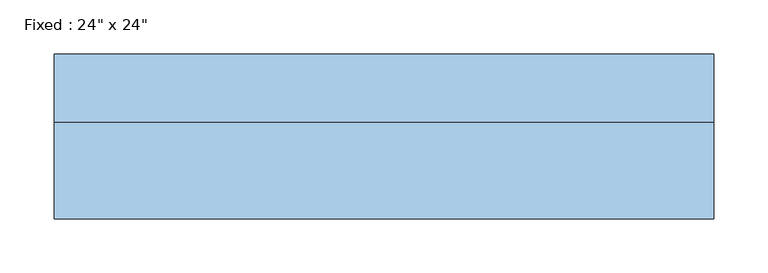
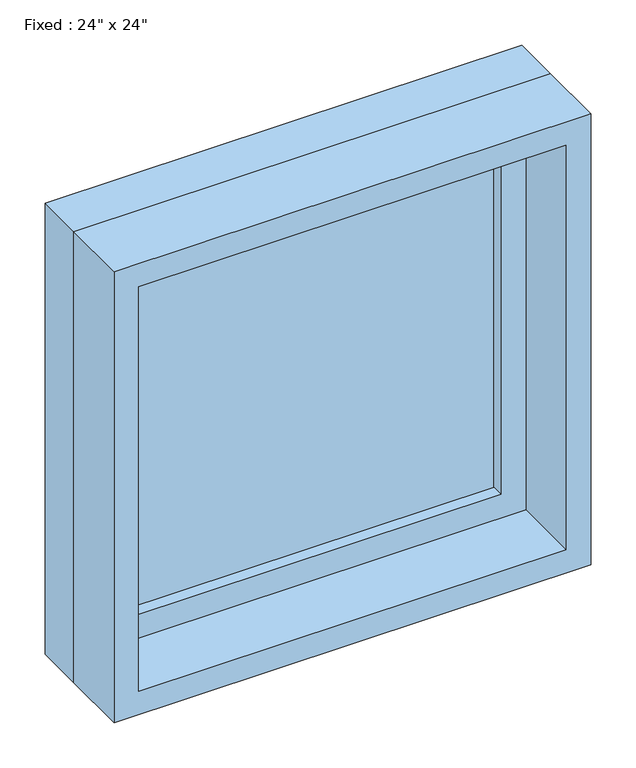
"""IFC4 building model written with IfcOpenShell, lengths in millimetres: window geometry."""

from ifc_helpers import new_model, si_unit, frame, origin, place, context, project, spatial, polyline, outline, extrude, source, transform, mapped, element, save


def window_aff1bc2a(model_context):
    return source(origin(), model_context, "Body", "SweptSolid", [
        extrude(outline(polyline([(203.2, 28.575), (-279.4, 28.575), (-279.4, 41.275), (203.2, 41.275), (203.2, 28.575)])), frame((0.0, 0.0, 977.9), z_axis=(0.0, 0.0, 1.0), x_axis=(1.0, 0.0, 0.0)), (0.0, 0.0, 1.0), 482.6),
        extrude(outline(polyline([(1504.95, -323.85), (933.45, -323.85), (933.45, 247.65), (1504.95, 247.65), (1504.95, -323.85)]), holes=[polyline([(1460.5, -279.4), (1460.5, 203.2), (977.9, 203.2), (977.9, -279.4), (1460.5, -279.4)])]), frame((0.0, 12.7, 0.0), z_axis=(0.0, 1.0, 0.0), x_axis=(0.0, 0.0, 1.0)), (0.0, 0.0, 1.0), 44.45),
        extrude(outline(polyline([(1524.0, -342.9), (914.4, -342.9), (914.4, 266.7), (1524.0, 266.7), (1524.0, -342.9)]), holes=[polyline([(1492.25, -311.15), (1492.25, 234.95), (946.15, 234.95), (946.15, -311.15), (1492.25, -311.15)])]), frame((0.0, -76.2, 0.0), z_axis=(0.0, 1.0, 0.0), x_axis=(0.0, 0.0, 1.0)), (0.0, 0.0, 1.0), 88.9),
        extrude(outline(polyline([(1524.0, 266.7), (1524.0, -342.9), (914.4, -342.9), (914.4, 266.7), (1524.0, 266.7)]), holes=[polyline([(1504.95, 247.65), (933.45, 247.65), (933.45, -323.85), (1504.95, -323.85), (1504.95, 247.65)])]), frame((0.0, 12.7, 0.0), z_axis=(0.0, 1.0, 0.0), x_axis=(0.0, 0.0, 1.0)), (0.0, 0.0, 1.0), 63.5),
    ])


if __name__ == "__main__":
    model = new_model("IFC4")
    model_context = context("Model", 3, world=origin())
    ifc_project = project(units=[si_unit("LENGTHUNIT", "METRE", prefix="MILLI")], contexts=[model_context])
    site = spatial("IfcSite", under=ifc_project)
    building = spatial("IfcBuilding", under=site)
    placement = place(None, origin())
    window_shape = window_aff1bc2a(model_context)
    element("IfcWindow", 1, ObjectType="Fixed : 24\" x 24\"", at=placement, inside=building, context=model_context, shape_type="MappedRepresentation", body=[
        mapped(window_shape, transform((0.0, 0.0, 0.0), x_axis=(1.0, 0.0, 0.0), y_axis=(0.0, 1.0, 0.0), z_axis=(0.0, 0.0, 1.0))),
    ])
    save(model, "model.ifc")

# Revit data of these elements
# Type "Fixed : 24\" x 24\""
#   Type Mark = "3"
#   Construction Type Id = "GSP4R"
#   Assembly Code = "B2020100"
#   Analytic Construction = "1/8 in Pilkington single glazing"
#   Visual Light Transmittance = 0.9
#   Solar Heat Gain Coefficient = 0.78
#   Heat Transfer Coefficient (U) = 0.6496 BTU/(h·ft²·°F)
#   Height = 2' - 0"
#   Default Sill Height = 3' - 0"
#   Width = 2' - 0"
#   Window Inset = 0' - 0 3/4"
#   Define Thermal Properties by = 1
#   Glass Pane Material = Glass
#   Sash Material = Sash
#   Wall Closure = (empty or 0)
# Element 1 (IfcWindow, "Fixed : 24\" x 24\"")
#   Materials on its faces: "Sash", "Glass"
# Materials
#   "Glass": class "Glass", colour RGB 0 128 192, transparency 0.75, Description = "Soda Lime Glass", Cost = 0
#   "Sash": class "Wood", colour RGB 224 178 126, transparency 0
